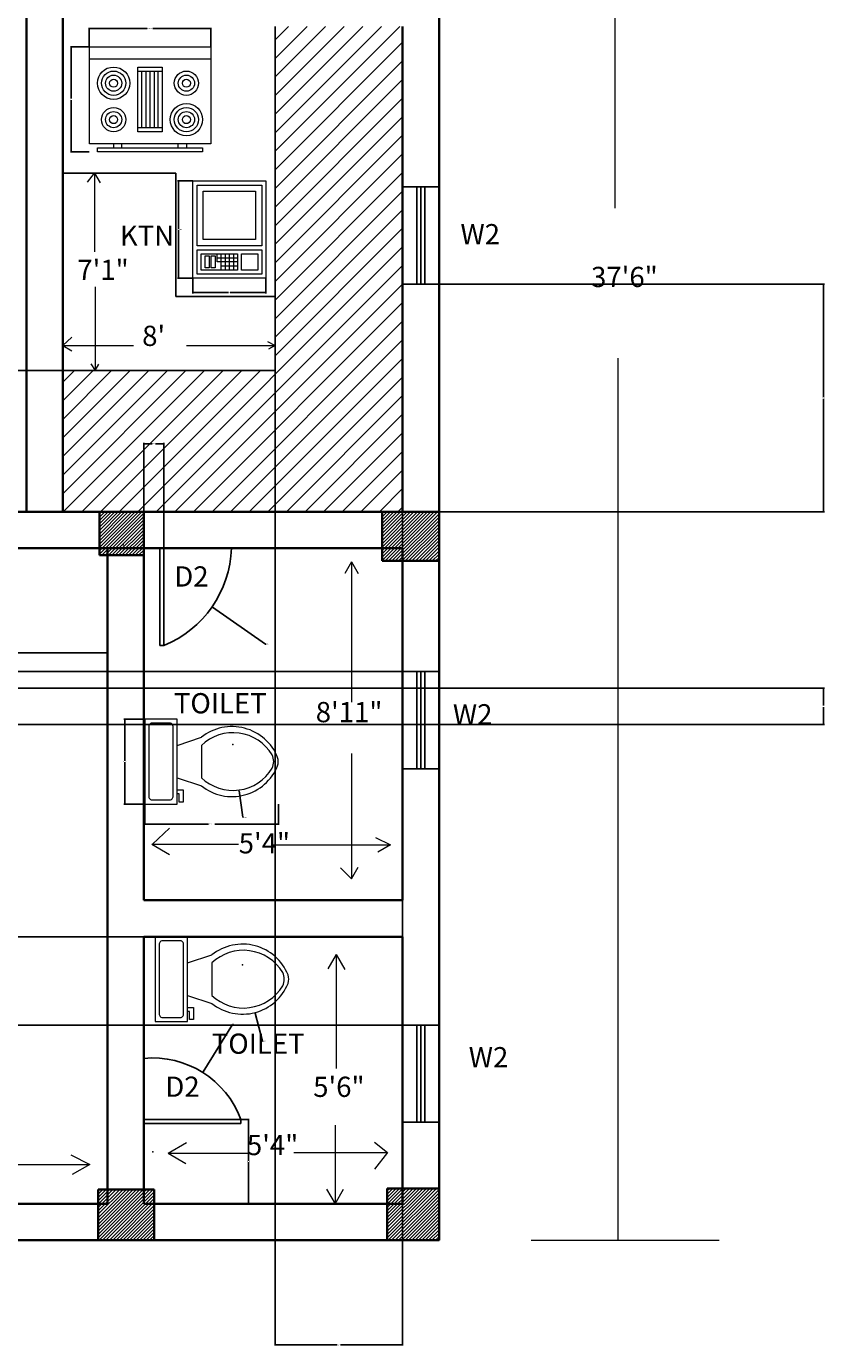
# Model space of a CAD drawing. Units: inches. Extents: x -4 to 429, y -457 to 84.
# Tile 3 of 4: x 232 to 429, y -457 to -131. Entities that reach past the tile are written whole.
import ezdxf

# ---------------------------------------------------------------- set-up
doc = ezdxf.new("R2010")
doc.units = ezdxf.units.IN
doc.header["$MEASUREMENT"] = 0
for name, color, linetype, lineweight in [('A-ANNO-DIMS', 2, 'Continuous', 18), ('A-ANNO-TEXT', 3, 'Continuous', 18), ('A-AREA-IDEN', 7, 'Continuous', 25), ('A-COLS', 7, 'Continuous', 35), ('A-COLS-PATT', 252, 'Continuous', 13), ('A-DOOR', 3, 'Continuous', 25), ('A-EQPM', 8, 'Continuous', 18), ('A-FLOR-CASE', 9, 'Continuous', 25), ('A-FLOR-CASE-PATT', 252, 'Continuous', 13), ('A-FLOR-FIXT', 9, 'Continuous', 18), ('A-GLAZ', 4, 'Continuous', 25), ('A-WALL', 7, 'Continuous', 35)]:
    doc.layers.add(name, color=color, linetype=linetype, lineweight=lineweight)
doc.styles.get("Standard").update_dxf_attribs({"font": 'arial.ttf'})
doc.dimstyles.get("Standard").update_dxf_attribs({"dimtxt": 0.18, "dimasz": 0.18, "dimexe": 0.18, "dimexo": 0.0625, "dimgap": 0.09, "dimtad": 0, "dimtih": 1, "dimtoh": 1, "dimdec": 4, "dimzin": 0, "dimdsep": 46, "dimtxsty": 'Standard', "dimcen": 0.09, "dimadec": 0, "dimazin": 0, "dimtfac": 1, "dimtdec": 4, "dimtofl": 0, "dimtmove": 0, "dimatfit": 3, "dimfxl": 1, "dimtolj": 1, "dimtzin": 0, "dimarcsym": 0})
pattern_1 = [(45, (-1330.13025, -719.5531), (-0.41542523, 0.41542523), [])]

# ---------------------------------------------------------------- blocks, each defined once
blk = doc.blocks.new('Microwave')
for p, q in [((18, 10), (22, 10)), ((19, 7), (19, 11)), ((20, 11), (20, 7)), ((21, 7), (21, 11)), ((22, 9), (18, 9)), ((18, 8), (22, 8)), ((22, 7), (18, 7)), ((19, 6), (19, 7)), ((20, 7), (20, 6)), ((20, 6), (18, 6))]:
    blk.add_line(p, q)
for points in [[(0, 0), (0, 18), (24, 18), (24, 0)], [(1, 1), (1, 17), (16, 17), (16, 1)], [(17, 1), (17, 17), (23, 17), (23, 1)], [(2.5, 2.5), (2.5, 15.5), (14.5, 15.5), (14.5, 2.5)], [(18, 12), (18, 16), (22, 16), (22, 12)], [(18, 2), (18, 11), (22, 11), (22, 2)], [(18.5, 4.5), (18.5, 5.5), (21.5, 5.5), (21.5, 4.5)], [(18.5, 3), (18.5, 4), (21.5, 4), (21.5, 3)]]:
    blk.add_lwpolyline(points, close=True)
blk = doc.blocks.new('Range-Oven - 30 in top')
for p, q in [((0, -3), (30, -3)), ((12, -6), (18, -6)), ((13, -20), (13, -6)), ((14, -6), (14, -20)), ((15, -20), (15, -6)), ((16, -6), (16, -20)), ((17, -20), (17, -6)), ((18, -20), (12, -20)), ((6, -24), (6, -25)), ((8, -25), (8, -24)), ((22, -25), (22, -24)), ((24, -24), (24, -25))]:
    blk.add_line(p, q)
for points in [[(0, -24), (0, 0), (30, 0), (30, -24)], [(12, -21), (12, -5), (18, -5), (18, -21)], [(2, -26), (2, -25), (28, -25), (28, -26)]]:
    blk.add_lwpolyline(points, close=True)
for centre, radius in [((6, -9), 4), ((6, -9), 3), ((24, -9), 3), ((6, -9), 2), ((6, -9), 1), ((24, -9), 2), ((24, -9), 1), ((6, -18), 3), ((6, -18), 2), ((24, -18), 4), ((24, -18), 3), ((24, -18), 2), ((6, -18), 1), ((24, -18), 1)]:
    blk.add_circle(centre, radius)
blk = doc.blocks.new('Toilet - top')
for p, q in [((9.5, -6), (9.5, -2)), ((-10, -8.5), (-8, -8.5)), ((-10, -9.5), (-10, -8.5)), ((-7, -9.5), (-10, -9.5)), ((-8, -8.5), (-8, -8)), ((-7, -8), (-7, -9.5)), ((-4, -8), (-6, -14)), ((4, -8), (6, -14)), ((4, -14), (-4, -14))]:
    blk.add_line(p, q)
blk.add_lwpolyline([(10.5, -8), (10.5, 0), (-10.5, 0), (-10.5, -8)], close=True)
for points in [[(-9.5, -2), (-9.5, -6)], [(8.5, -1), (-8.5, -1)], [(-8.5, -7), (8.5, -7)]]:
    blk.add_lwpolyline(points)
for centre, radius, start, end in [((-8.62, -1.88), 0.884, 81.8699, 188.1301), ((8.62, -1.88), 0.884, 351.8699, 98.1301), ((-8.62, -6.12), 0.884, 171.8699, 278.1301), ((8.62, -6.12), 0.884, 261.8699, 8.1301), ((3.52, -21.58), 12.17, 141.4691, 247.9714), ((4.2, -21.82), 11.33, 136.3677, 238.9468), ((-3.52, -21.58), 12.17, 292.0284, 38.5307), ((-4.2, -21.82), 11.33, 301.053, 43.6321), ((0, -27.88), 4, 245.7318, 294.2682), ((0, -29), 4, 254.8605, 285.1395)]:
    blk.add_arc(centre, radius, start, end)
blk = doc.blocks.new('WIN-24IN-9IN-WALL')
for p, q in [((0, 5.5), (24, 5.5)), ((0, 4.5), (24, 4.5)), ((0, 3.5), (24, 3.5))]:
    blk.add_line(p, q)
blk.add_lwpolyline([(0, 9), (24, 9), (24, 0), (0, 0)], close=True)
blk = doc.blocks.new('DOOR-LEAF-24IN')
for p, q in [((0, 0), (0, 24)), ((0, 24), (1, 24)), ((1, 24), (1, 0))]:
    blk.add_line(p, q)
blk = doc.blocks.new('*D20')
at = {"layer": 'A-ANNO-DIMS', "color": 0, "lineweight": -2, "transparency": 16777216}
for p, q in [((261.3, -323.62), (261.3, -328.69)), ((294.34, -323.62), (294.34, -328.69)), ((261.48, -328.51), (277.04, -328.51)), ((294.16, -328.51), (278.59, -328.51))]:
    blk.add_line(p, q, dxfattribs=at)
at = {"layer": 'A-ANNO-DIMS', "color": 0, "transparency": 16777216}
for points in [[(261.48, -328.48), (261.48, -328.54), (261.3, -328.51)], [(294.16, -328.48), (294.16, -328.54), (294.34, -328.51)]]:
    blk.add_solid(points, dxfattribs=at)
at = {"layer": 'Defpoints', "color": 0, "transparency": 16777216}
for p in [(261.3, -323.55), (294.34, -323.55), (261.3, -328.51)]:
    blk.add_point(p, dxfattribs=at)
at = {"layer": 'A-ANNO-DIMS', "color": 0, "transparency": 16777216, "insert": (277.82, -328.51), "char_height": 0.18, "attachment_point": 5}
blk.add_mtext('\\A1;WC 33 TYP.', dxfattribs=at)
blk = doc.blocks.new('*D21')
at = {"layer": 'A-ANNO-DIMS', "color": 0, "lineweight": -2, "transparency": 16777216}
for p, q in [((261.23, -302.55), (256.16, -302.55)), ((256.34, -302.73), (256.34, -312.87)), ((256.34, -323.37), (256.34, -313.24)), ((261.23, -323.55), (256.16, -323.55))]:
    blk.add_line(p, q, dxfattribs=at)
at = {"layer": 'A-ANNO-DIMS', "color": 0, "transparency": 16777216}
for points in [[(256.31, -302.73), (256.37, -302.73), (256.34, -302.55)], [(256.31, -323.37), (256.37, -323.37), (256.34, -323.55)]]:
    blk.add_solid(points, dxfattribs=at)
at = {"layer": 'Defpoints', "color": 0, "transparency": 16777216}
for p in [(256.34, -302.55), (261.3, -302.55), (261.3, -323.55)]:
    blk.add_point(p, dxfattribs=at)
at = {"layer": 'A-ANNO-DIMS', "color": 0, "transparency": 16777216, "insert": (256.34, -313.05), "char_height": 0.18, "attachment_point": 5}
blk.add_mtext('\\A1;21 TYP.', dxfattribs=at)
blk = doc.blocks.new('*D28')
at = {"layer": 'A-ANNO-DIMS', "color": 0, "lineweight": -2, "transparency": 16777216}
for p, q in [((273.16, -169.55), (269.44, -169.55)), ((269.62, -169.73), (269.62, -181.37)), ((269.62, -193.37), (269.62, -181.74)), ((273.16, -193.55), (269.44, -193.55))]:
    blk.add_line(p, q, dxfattribs=at)
at = {"layer": 'A-ANNO-DIMS', "color": 0, "transparency": 16777216}
for points in [[(269.59, -169.73), (269.65, -169.73), (269.62, -169.55)], [(269.59, -193.37), (269.65, -193.37), (269.62, -193.55)]]:
    blk.add_solid(points, dxfattribs=at)
at = {"layer": 'Defpoints', "color": 0, "transparency": 16777216}
for p in [(273.22, -169.55), (269.62, -193.55), (273.22, -193.55)]:
    blk.add_point(p, dxfattribs=at)
at = {"layer": 'A-ANNO-DIMS', "color": 0, "transparency": 16777216, "insert": (269.62, -181.55), "char_height": 0.18, "attachment_point": 5}
blk.add_mtext('\\A1;MICROWAVE 24', dxfattribs=at)
blk = doc.blocks.new('*D29')
at = {"layer": 'A-ANNO-DIMS', "color": 0, "lineweight": -2, "transparency": 16777216}
for p, q in [((273.22, -193.62), (273.22, -197.33)), ((291.22, -193.62), (291.22, -197.33)), ((273.4, -197.15), (282.01, -197.15)), ((291.04, -197.15), (282.43, -197.15))]:
    blk.add_line(p, q, dxfattribs=at)
at = {"layer": 'A-ANNO-DIMS', "color": 0, "transparency": 16777216}
for points in [[(273.4, -197.12), (273.4, -197.18), (273.22, -197.15)], [(291.04, -197.12), (291.04, -197.18), (291.22, -197.15)]]:
    blk.add_solid(points, dxfattribs=at)
at = {"layer": 'Defpoints', "color": 0, "transparency": 16777216}
for p in [(273.22, -193.55), (291.22, -193.55), (291.22, -197.15)]:
    blk.add_point(p, dxfattribs=at)
at = {"layer": 'A-ANNO-DIMS', "color": 0, "transparency": 16777216, "insert": (282.22, -197.15), "char_height": 0.18, "attachment_point": 5}
blk.add_mtext('\\A1;18', dxfattribs=at)
blk = doc.blocks.new('*D30')
at = {"layer": 'A-ANNO-DIMS', "color": 0, "lineweight": -2, "transparency": 16777216}
for p, q in [((247.6, -136.32), (247.6, -131.7)), ((247.78, -131.88), (261.91, -131.88)), ((277.42, -131.88), (263.3, -131.88)), ((277.6, -136.32), (277.6, -131.7))]:
    blk.add_line(p, q, dxfattribs=at)
at = {"layer": 'A-ANNO-DIMS', "color": 0, "transparency": 16777216}
for points in [[(247.78, -131.85), (247.78, -131.91), (247.6, -131.88)], [(277.42, -131.85), (277.42, -131.91), (277.6, -131.88)]]:
    blk.add_solid(points, dxfattribs=at)
at = {"layer": 'Defpoints', "color": 0, "transparency": 16777216}
for p in [(277.6, -131.88), (247.6, -136.38), (277.6, -136.38)]:
    blk.add_point(p, dxfattribs=at)
at = {"layer": 'A-ANNO-DIMS', "color": 0, "transparency": 16777216, "insert": (262.6, -131.88), "char_height": 0.18, "attachment_point": 5}
blk.add_mtext('\\A1;RANGE 30', dxfattribs=at)
blk = doc.blocks.new('*D31')
at = {"layer": 'A-ANNO-DIMS', "color": 0, "lineweight": -2, "transparency": 16777216}
for p, q in [((247.54, -136.38), (242.92, -136.38)), ((243.1, -136.56), (243.1, -149.2)), ((243.1, -162.2), (243.1, -149.57)), ((247.54, -162.38), (242.92, -162.38))]:
    blk.add_line(p, q, dxfattribs=at)
at = {"layer": 'A-ANNO-DIMS', "color": 0, "transparency": 16777216}
for points in [[(243.07, -136.56), (243.13, -136.56), (243.1, -136.38)], [(243.07, -162.2), (243.13, -162.2), (243.1, -162.38)]]:
    blk.add_solid(points, dxfattribs=at)
at = {"layer": 'Defpoints', "color": 0, "transparency": 16777216}
for p in [(243.1, -136.38), (247.6, -136.38), (247.6, -162.38)]:
    blk.add_point(p, dxfattribs=at)
at = {"layer": 'A-ANNO-DIMS', "color": 0, "transparency": 16777216, "insert": (243.1, -149.38), "char_height": 0.18, "attachment_point": 5}
blk.add_mtext('\\A1;26', dxfattribs=at)
blk = doc.blocks.new('*D33')
at = {"layer": 'A-ANNO-DIMS', "color": 0, "lineweight": -2, "transparency": 16777216}
for p, q in [((70.12, -294.9), (429.31, -294.9)), ((429.13, -295.08), (429.13, -299.22)), ((429.13, -303.72), (429.13, -299.59)), ((70.12, -303.9), (429.31, -303.9))]:
    blk.add_line(p, q, dxfattribs=at)
at = {"layer": 'A-ANNO-DIMS', "color": 0, "transparency": 16777216}
for points in [[(429.1, -295.08), (429.16, -295.08), (429.13, -294.9)], [(429.1, -303.72), (429.16, -303.72), (429.13, -303.9)]]:
    blk.add_solid(points, dxfattribs=at)
at = {"layer": 'Defpoints', "color": 0, "transparency": 16777216}
for p in [(70.06, -294.9), (70.06, -303.9), (429.13, -303.9)]:
    blk.add_point(p, dxfattribs=at)
at = {"layer": 'A-ANNO-DIMS', "color": 0, "transparency": 16777216, "insert": (429.13, -299.4), "char_height": 0.18, "attachment_point": 5}
blk.add_mtext('\\A1;9', dxfattribs=at)
blk = doc.blocks.new('*D36')
at = {"layer": 'A-ANNO-DIMS', "color": 0, "lineweight": -2, "transparency": 16777216}
for p, q in [((293.52, -131.4), (293.52, -457.42)), ((325.06, -131.4), (325.06, -457.42)), ((293.7, -457.24), (308.89, -457.24)), ((324.88, -457.24), (309.68, -457.24))]:
    blk.add_line(p, q, dxfattribs=at)
at = {"layer": 'A-ANNO-DIMS', "color": 0, "transparency": 16777216}
for points in [[(293.7, -457.21), (293.7, -457.27), (293.52, -457.24)], [(324.88, -457.21), (324.88, -457.27), (325.06, -457.24)]]:
    blk.add_solid(points, dxfattribs=at)
at = {"layer": 'Defpoints', "color": 0, "transparency": 16777216}
for p in [(293.52, -131.34), (325.06, -131.34), (325.06, -457.24)]:
    blk.add_point(p, dxfattribs=at)
at = {"layer": 'A-ANNO-DIMS', "color": 0, "transparency": 16777216, "insert": (309.29, -457.24), "char_height": 0.18, "attachment_point": 5}
blk.add_mtext('\\A1;31.54', dxfattribs=at)
blk = doc.blocks.new('*D37')
at = {"layer": 'A-ANNO-DIMS', "color": 0, "lineweight": -2, "transparency": 16777216}
for p, q in [((240.99, -216.42), (215.03, -216.42)), ((215.21, -216.6), (215.21, -233.7)), ((215.21, -251.16), (215.21, -234.06)), ((240.99, -251.34), (215.03, -251.34))]:
    blk.add_line(p, q, dxfattribs=at)
at = {"layer": 'A-ANNO-DIMS', "color": 0, "transparency": 16777216}
for points in [[(215.18, -216.6), (215.24, -216.6), (215.21, -216.42)], [(215.18, -251.16), (215.24, -251.16), (215.21, -251.34)]]:
    blk.add_solid(points, dxfattribs=at)
at = {"layer": 'Defpoints', "color": 0, "transparency": 16777216}
for p in [(215.21, -216.42), (241.06, -216.42), (241.06, -251.34)]:
    blk.add_point(p, dxfattribs=at)
at = {"layer": 'A-ANNO-DIMS', "color": 0, "transparency": 16777216, "insert": (215.21, -233.88), "char_height": 0.18, "attachment_point": 5}
blk.add_mtext('\\A1;34.92', dxfattribs=at)
blk = doc.blocks.new('*D40')
at = {"layer": 'A-ANNO-DIMS', "color": 0, "lineweight": -2, "transparency": 16777216}
for p, q in [((334.12, -195.04), (429.31, -195.04)), ((429.13, -195.22), (429.13, -223.01)), ((429.13, -251.16), (429.13, -223.37)), ((334.12, -251.34), (429.31, -251.34))]:
    blk.add_line(p, q, dxfattribs=at)
at = {"layer": 'A-ANNO-DIMS', "color": 0, "transparency": 16777216}
for points in [[(429.1, -195.22), (429.16, -195.22), (429.13, -195.04)], [(429.1, -251.16), (429.16, -251.16), (429.13, -251.34)]]:
    blk.add_solid(points, dxfattribs=at)
at = {"layer": 'Defpoints', "color": 0, "transparency": 16777216}
for p in [(334.06, -195.04), (334.06, -251.34), (429.13, -251.34)]:
    blk.add_point(p, dxfattribs=at)
at = {"layer": 'A-ANNO-DIMS', "color": 0, "transparency": 16777216, "insert": (429.13, -223.19), "char_height": 0.18, "attachment_point": 5}
blk.add_mtext('\\A1;56.3', dxfattribs=at)
blk = doc.blocks.new('*D41')
at = {"layer": 'A-ANNO-DIMS', "color": 0, "lineweight": -2, "transparency": 16777216}
for p, q in [((324.99, -260.34), (-3.97, -260.34)), ((-3.79, -260.52), (-3.79, -275.4)), ((-3.79, -290.65), (-3.79, -275.76)), ((324.99, -290.83), (-3.97, -290.83))]:
    blk.add_line(p, q, dxfattribs=at)
at = {"layer": 'A-ANNO-DIMS', "color": 0, "transparency": 16777216}
for points in [[(-3.82, -260.52), (-3.76, -260.52), (-3.79, -260.34)], [(-3.82, -290.65), (-3.76, -290.65), (-3.79, -290.83)]]:
    blk.add_solid(points, dxfattribs=at)
at = {"layer": 'Defpoints', "color": 0, "transparency": 16777216}
for p in [(325.06, -260.34), (-3.79, -290.83), (325.06, -290.83)]:
    blk.add_point(p, dxfattribs=at)
at = {"layer": 'A-ANNO-DIMS', "color": 0, "transparency": 16777216, "insert": (-3.79, -275.58), "char_height": 0.18, "attachment_point": 5}
blk.add_mtext('\\A1;30.486', dxfattribs=at)
blk = doc.blocks.new('*D42')
at = {"layer": 'A-ANNO-DIMS', "color": 0, "lineweight": -2, "transparency": 16777216}
for p, q in [((324.99, -356.34), (-3.97, -356.34)), ((-3.79, -356.52), (-3.79, -367.09)), ((-3.79, -378.03), (-3.79, -367.46)), ((324.99, -378.21), (-3.97, -378.21))]:
    blk.add_line(p, q, dxfattribs=at)
at = {"layer": 'A-ANNO-DIMS', "color": 0, "transparency": 16777216}
for points in [[(-3.82, -356.52), (-3.76, -356.52), (-3.79, -356.34)], [(-3.82, -378.03), (-3.76, -378.03), (-3.79, -378.21)]]:
    blk.add_solid(points, dxfattribs=at)
at = {"layer": 'Defpoints', "color": 0, "transparency": 16777216}
for p in [(325.06, -356.34), (-3.79, -378.21), (325.06, -378.21)]:
    blk.add_point(p, dxfattribs=at)
at = {"layer": 'A-ANNO-DIMS', "color": 0, "transparency": 16777216, "insert": (-3.79, -367.28), "char_height": 0.18, "attachment_point": 5}
blk.add_mtext('\\A1;21.87', dxfattribs=at)
blk = doc.blocks.new('*D48')
at = {"layer": 'A-ANNO-DIMS', "color": 0, "lineweight": -2, "transparency": 16777216}
for p, q in [((130.63, -260.4), (130.63, -286.37)), ((252.06, -260.4), (252.06, -286.37)), ((130.81, -286.19), (190.89, -286.19)), ((251.88, -286.19), (191.8, -286.19))]:
    blk.add_line(p, q, dxfattribs=at)
at = {"layer": 'A-ANNO-DIMS', "color": 0, "transparency": 16777216}
for points in [[(130.81, -286.16), (130.81, -286.22), (130.63, -286.19)], [(251.88, -286.16), (251.88, -286.22), (252.06, -286.19)]]:
    blk.add_solid(points, dxfattribs=at)
at = {"layer": 'Defpoints', "color": 0, "transparency": 16777216}
for p in [(130.63, -260.34), (252.06, -260.34), (130.63, -286.19)]:
    blk.add_point(p, dxfattribs=at)
at = {"layer": 'A-ANNO-DIMS', "color": 0, "transparency": 16777216, "insert": (191.35, -286.19), "char_height": 0.18, "attachment_point": 5}
blk.add_mtext('\\A1;121.42', dxfattribs=at)
blk = doc.blocks.new('*D49')
at = {"layer": 'A-ANNO-DIMS', "color": 0, "lineweight": -2, "transparency": 16777216}
for p, q in [((261.06, -260.28), (261.06, -234.31)), ((261.24, -234.49), (263.14, -234.49)), ((265.84, -234.49), (263.94, -234.49)), ((266.02, -260.28), (266.02, -234.31))]:
    blk.add_line(p, q, dxfattribs=at)
at = {"layer": 'A-ANNO-DIMS', "color": 0, "transparency": 16777216}
for points in [[(261.24, -234.46), (261.24, -234.52), (261.06, -234.49)], [(265.84, -234.46), (265.84, -234.52), (266.02, -234.49)]]:
    blk.add_solid(points, dxfattribs=at)
at = {"layer": 'Defpoints', "color": 0, "transparency": 16777216}
for p in [(266.02, -234.49), (261.06, -260.34), (266.02, -260.34)]:
    blk.add_point(p, dxfattribs=at)
at = {"layer": 'A-ANNO-DIMS', "color": 0, "transparency": 16777216, "insert": (263.54, -234.49), "char_height": 0.18, "attachment_point": 5}
blk.add_mtext('\\A1;4.964', dxfattribs=at)
blk = doc.blocks.new('*D50')
at = {"layer": 'A-ANNO-DIMS', "color": 0, "lineweight": -2, "transparency": 16777216}
for p, q in [((261.12, -401.49), (287.09, -401.49)), ((286.91, -401.67), (286.91, -411.73)), ((286.91, -422.16), (286.91, -412.1)), ((261.12, -422.34), (287.09, -422.34))]:
    blk.add_line(p, q, dxfattribs=at)
at = {"layer": 'A-ANNO-DIMS', "color": 0, "transparency": 16777216}
for points in [[(286.88, -401.67), (286.94, -401.67), (286.91, -401.49)], [(286.88, -422.16), (286.94, -422.16), (286.91, -422.34)]]:
    blk.add_solid(points, dxfattribs=at)
at = {"layer": 'Defpoints', "color": 0, "transparency": 16777216}
for p in [(261.06, -401.49), (261.06, -422.34), (286.91, -422.34)]:
    blk.add_point(p, dxfattribs=at)
at = {"layer": 'A-ANNO-DIMS', "color": 0, "transparency": 16777216, "insert": (286.91, -411.92), "char_height": 0.18, "attachment_point": 5}
blk.add_mtext('\\A1;20.848', dxfattribs=at)
blk = doc.blocks.new('*D57')
at = {"layer": 'A-ANNO-DIMS', "color": 0, "lineweight": -2, "transparency": 16777216}
for p, q in [((255.86, -259.49), (256.04, -259.49)), ((255.95, -259.58), (255.95, -259.4)), ((291.14, -284.02), (278.09, -274.92)), ((291.32, -284.02), (291.14, -284.02))]:
    blk.add_line(p, q, dxfattribs=at)
at = {"layer": 'A-ANNO-DIMS', "color": 0, "transparency": 16777216}
blk.add_solid([(278.11, -274.9), (278.07, -274.95), (277.94, -274.82)], dxfattribs=at)
at = {"layer": 'Defpoints', "color": 0, "transparency": 16777216}
for p in [(255.95, -259.49), (277.94, -274.82)]:
    blk.add_point(p, dxfattribs=at)
at = {"layer": 'A-ANNO-DIMS', "color": 0, "transparency": 16777216, "insert": (291.79, -284.02), "char_height": 0.18, "attachment_point": 5}
blk.add_mtext('\\A1;R26.81', dxfattribs=at)
blk = doc.blocks.new('*D58')
at = {"layer": 'A-ANNO-DIMS', "color": 0, "lineweight": -2, "transparency": 16777216}
for p, q in [((283.03, -378.07), (275.72, -389.72)), ((283.21, -378.07), (283.03, -378.07)), ((263.18, -409.54), (263.36, -409.54)), ((263.27, -409.63), (263.27, -409.45))]:
    blk.add_line(p, q, dxfattribs=at)
at = {"layer": 'A-ANNO-DIMS', "color": 0, "transparency": 16777216}
blk.add_solid([(275.69, -389.7), (275.74, -389.74), (275.62, -389.87)], dxfattribs=at)
at = {"layer": 'Defpoints', "color": 0, "transparency": 16777216}
for p in [(275.62, -389.87), (263.27, -409.54)]:
    blk.add_point(p, dxfattribs=at)
at = {"layer": 'A-ANNO-DIMS', "color": 0, "transparency": 16777216, "insert": (283.69, -378.07), "char_height": 0.18, "attachment_point": 5}
blk.add_mtext('\\A1;R23.23', dxfattribs=at)
blk = doc.blocks.new('*D62')
at = {"layer": 'A-ANNO-DIMS', "color": 0, "lineweight": -2, "transparency": 16777216}
for p, q in [((285.38, -363.32), (285.56, -363.32)), ((285.47, -363.41), (285.47, -363.23)), ((290.41, -382.15), (288.6, -375.26)), ((290.59, -382.15), (290.41, -382.15))]:
    blk.add_line(p, q, dxfattribs=at)
at = {"layer": 'A-ANNO-DIMS', "color": 0, "transparency": 16777216}
blk.add_solid([(288.63, -375.26), (288.58, -375.27), (288.56, -375.09)], dxfattribs=at)
at = {"layer": 'Defpoints', "color": 0, "transparency": 16777216}
for p in [(285.47, -363.32), (288.56, -375.09)]:
    blk.add_point(p, dxfattribs=at)
at = {"layer": 'A-ANNO-DIMS', "color": 0, "transparency": 16777216, "insert": (291.27, -382.15), "char_height": 0.18, "attachment_point": 5}
blk.add_mtext('\\A1;4X R12.17', dxfattribs=at)
blk = doc.blocks.new('*D63')
at = {"layer": 'A-ANNO-DIMS', "color": 0, "lineweight": -2, "transparency": 16777216}
for p, q in [((283.02, -308.85), (283.2, -308.85)), ((283.11, -308.94), (283.11, -308.76)), ((285.53, -326.82), (284.65, -320.26)), ((285.71, -326.82), (285.53, -326.82))]:
    blk.add_line(p, q, dxfattribs=at)
at = {"layer": 'A-ANNO-DIMS', "color": 0, "transparency": 16777216}
blk.add_solid([(284.68, -320.26), (284.62, -320.27), (284.62, -320.08)], dxfattribs=at)
at = {"layer": 'Defpoints', "color": 0, "transparency": 16777216}
for p in [(283.11, -308.85), (284.62, -320.08)]:
    blk.add_point(p, dxfattribs=at)
at = {"layer": 'A-ANNO-DIMS', "color": 0, "transparency": 16777216, "insert": (286.39, -326.82), "char_height": 0.18, "attachment_point": 5}
blk.add_mtext('\\A1;4X R11.33', dxfattribs=at)

msp = doc.modelspace()

# ---------------------------------------------------------------- hatches: boundary and pattern name
at = {"layer": 'A-COLS-PATT'}
h = msp.add_hatch(dxfattribs=at)
h.set_pattern_fill('ANSI31', color=256, scale=4.7)
h.set_pattern_definition(pattern_1)
h.paths.add_polyline_path([(334.0572, -251.3399), (325.0572, -251.3399), (319.9964, -251.3399), (319.9964, -260.3399), (325.0572, -260.3399), (325.0572, -263.4636), (334.0572, -263.4636)])
h.paths.add_polyline_path([(325.0572, -260.3399), (319.9964, -260.3399), (319.9964, -263.4636), (325.0572, -263.4636)], flags=17)
h.paths.add_polyline_path([(34.0899, -251.3399), (31.0572, -251.3399), (22.0572, -251.3399), (22.0572, -263.5568), (31.0572, -263.5568), (31.0572, -260.3399), (34.0899, -260.3399)])
h.paths.add_polyline_path([(34.0899, -260.3399), (31.0572, -260.3399), (31.0572, -263.5568), (34.0899, -263.5568)], flags=17)
h = msp.add_hatch(dxfattribs=at)
h.set_pattern_fill('ANSI31', color=256, scale=4.7)
h.set_pattern_definition(pattern_1)
h.paths.add_polyline_path([(261.0572, -251.3399), (250.1046, -251.3399), (250.1046, -260.3399), (261.0572, -260.3399)])
h.paths.add_polyline_path([(252.0572, -260.3399), (250.1046, -260.3399), (250.1046, -262.0762), (252.0572, -262.0762)])
h.paths.add_polyline_path([(261.0572, -260.3399), (252.0572, -260.3399), (252.0572, -262.0762), (261.0572, -262.0762)])
h = msp.add_hatch(dxfattribs=at)
h.set_pattern_fill('ANSI31', color=256, scale=4.7)
h.set_pattern_definition(pattern_1)
h.paths.add_polyline_path([(263.6379, -422.3399), (261.0572, -422.3399), (261.0572, -418.8132), (252.0572, -418.8132), (252.0572, -422.3399), (249.7857, -422.3399), (249.7857, -431.3399), (263.6379, -431.3399)])
h.paths.add_polyline_path([(252.0572, -418.8132), (249.7857, -418.8132), (249.7857, -422.3399), (252.0572, -422.3399)], flags=17)
h.paths.add_polyline_path([(263.6379, -418.8132), (261.0572, -418.8132), (261.0572, -422.3399), (263.6379, -422.3399)], flags=17)
h = msp.add_hatch(dxfattribs=at)
h.set_pattern_fill('ANSI31', color=256, scale=4.7)
h.set_pattern_definition(pattern_1)
h.paths.add_polyline_path([(325.0572, -418.5798), (321.2689, -418.5798), (321.2689, -422.3399), (325.0572, -422.3399)], flags=17)
h.paths.add_polyline_path([(334.0572, -418.5798), (325.0572, -418.5798), (325.0572, -422.3399), (321.2689, -422.3399), (321.2689, -431.3399), (334.0572, -431.3399)])
at = {"layer": 'A-FLOR-CASE-PATT'}
h = msp.add_hatch(dxfattribs=at)
h.set_pattern_fill('ANSI31', color=256, scale=26)
h.set_pattern_definition([(45, (-1330.1303, -719.553), (-2.298097, 2.298097), [])])
h.paths.add_polyline_path([(325.0572, -131.3399), (293.5167, -131.3399), (293.5167, -216.4188), (241.0572, -216.4188), (241.0572, -251.3399), (325.0572, -251.3399)])

# ---------------------------------------------------------------- linework, layer by layer
at = {"layer": 'A-ANNO-DIMS'}
for p, q in [((377.4887, 18.6601), (377.4887, -176.2694)), ((247.1193, -169.8571), (248.9197, -167.5973)), ((248.9197, -167.5973), (248.9197, -187.0745)), ((248.9197, -167.5973), (250.3069, -169.9999)), ((249.0695, -195.7353), (249.0695, -216.4188)), ((243.2479, -208.1928), (241.0572, -210.2098)), ((241.0572, -210.2098), (258.5297, -210.2098)), ((241.0572, -210.2098), (243.3025, -211.5061)), ((271.5893, -210.2098), (293.5167, -210.2098)), ((291.6293, -209.2601), (293.5167, -210.2098)), ((293.5167, -210.2098), (291.88, -211.1548)), ((247.9929, -214.7252), (249.0695, -216.4188)), ((249.0695, -216.4188), (249.9759, -214.8489)), ((378.2756, -213.3463), (378.2756, -431.3399)), ((312.4369, -263.6991), (310.7836, -266.5628)), ((312.4369, -263.6991), (312.4369, -298.3746)), ((312.4369, -263.6991), (314.0927, -266.567)), ((312.4369, -311.0802), (312.4369, -342.0499)), ((263.1937, -333.4878), (267.3935, -329.4934)), ((318.3203, -331.8236), (322.0243, -333.6537)), ((263.0687, -333.4878), (284.492, -333.4878)), ((263.0687, -333.4878), (267.4223, -336.0013)), ((292.6296, -333.6537), (322.0243, -333.6537)), ((322.0243, -333.6537), (318.9595, -335.4231)), ((309.701, -339.3156), (312.4369, -342.0499)), ((312.4369, -342.0499), (314.0884, -339.1895)), ((308.6569, -360.748), (306.6025, -364.3063)), ((308.6569, -360.748), (308.6569, -388.8905)), ((308.6569, -360.748), (310.7932, -364.4481)), ((308.386, -402.9617), (308.386, -422.3399)), ((267.062, -409.8655), (271.6342, -407.2257)), ((318.1218, -407.1378), (321.3323, -409.6606)), ((243.0363, -410.2286), (247.6925, -412.6439)), ((267.062, -409.8655), (286.861, -409.8655)), ((267.062, -409.8655), (271.4469, -412.3971)), ((298.1349, -409.6606), (321.3323, -409.6606)), ((321.3323, -409.6606), (318.1018, -413.7716)), ((198.9877, -412.6439), (247.6925, -412.6439)), ((247.6925, -412.6439), (243.3818, -415.1326)), ((306.2357, -418.7619), (308.386, -422.3399)), ((308.386, -422.3399), (310.4388, -418.7843)), ((356.7945, -431.3861), (403.2831, -431.3861))]:
    msp.add_line(p, q, dxfattribs=at)
at = {"layer": 'A-COLS'}
for p, q in [((261.0572, -251.3399), (250.1046, -251.3399)), ((250.1046, -251.3399), (250.1046, -262.0762)), ((261.0572, -260.3399), (261.0572, -251.3399)), ((319.9964, -263.4636), (319.9964, -251.3399)), ((325.0572, -251.3399), (334.0572, -251.3399)), ((250.1046, -262.0762), (261.0572, -262.0762)), ((319.9964, -263.4636), (334.0572, -263.4636)), ((249.7857, -431.3399), (249.7857, -418.8132)), ((249.7857, -418.8132), (263.6379, -418.8132)), ((263.6379, -418.8132), (263.6379, -431.3399)), ((334.0572, -418.5798), (321.2689, -418.5798)), ((321.2689, -418.5798), (321.2689, -431.3399))]:
    msp.add_line(p, q, dxfattribs=at)
at = {"layer": 'A-DOOR'}
for centre, radius, start, end in [((255.9463, -259.4939), 26.8112, 292.073261, 358.191774), ((263.2693, -409.5429), 23.2277, 20.279231, 95.464723)]:
    msp.add_arc(centre, radius, start, end, dxfattribs=at)
at = {"layer": 'A-FLOR-CASE'}
for p, q in [((293.5167, -131.3399), (293.5167, -216.4188)), ((241.0572, -167.5973), (268.9792, -167.5973)), ((268.9792, -167.5973), (268.9792, -198.1317)), ((268.9792, -198.1317), (293.5167, -198.1317)), ((293.5167, -216.4188), (241.0572, -216.4188))]:
    msp.add_line(p, q, dxfattribs=at)
at = {"layer": 'A-WALL'}
for p, q in [((232.0572, -251.3399), (232.0572, -122.3399)), ((241.0572, -251.3399), (241.0572, -122.3399)), ((325.0572, -131.3399), (325.0572, -251.3399)), ((31.0572, -251.3399), (325.0572, -251.3399)), ((31.0572, -260.3399), (325.0572, -260.3399)), ((252.0572, -260.3399), (252.0572, -422.3399)), ((261.0572, -260.3399), (261.0572, -347.3399)), ((325.0572, -260.3399), (325.0572, -347.3399)), ((325.0572, -347.3399), (261.0572, -347.3399)), ((325.0572, -356.3399), (261.0572, -356.3399)), ((261.0572, -356.3399), (261.0572, -422.3399)), ((325.0572, -356.3399), (325.0572, -422.3399)), ((252.0572, -422.3399), (118.0572, -422.3399)), ((325.0572, -422.3399), (261.0572, -422.3399))]:
    msp.add_line(p, q, dxfattribs=at)
msp.add_lwpolyline([(22.0572, 18.6601), (334.0572, 18.6601), (334.0572, -431.3399), (22.0572, -431.3399)], close=True, dxfattribs=at)

# ---------------------------------------------------------------- block references
at = {"layer": 'A-DOOR'}
for p, rotation in [((266.0219, -260.3398), 180), ((261.0571, -401.492), 270)]:
    msp.add_blockref('DOOR-LEAF-24IN', p, dxfattribs=dict(at, rotation=rotation))
at = {"layer": 'A-EQPM'}
msp.add_blockref('Range-Oven - 30 in top', (247.6038, -136.3834), dxfattribs=at)
at = {"layer": 'A-EQPM', "rotation": 270}
msp.add_blockref('Microwave', (273.2213, -169.5549), dxfattribs=at)
at = {"layer": 'A-FLOR-FIXT', "rotation": 90}
for p in [(261.2956, -313.0548), (263.8863, -366.8399)]:
    msp.add_blockref('Toilet - top', p, dxfattribs=at)
at = {"layer": 'A-GLAZ', "extrusion": (0, 0, -1), "zscale": -1, "rotation": 269.9999999999999}
for p in [(-334.0573, -171.0372), (-334.0573, -290.8262), (-334.0573, -378.2116)]:
    msp.add_blockref('WIN-24IN-9IN-WALL', p, dxfattribs=at)

# ---------------------------------------------------------------- texts
at = {"layer": 'A-ANNO-DIMS', "char_height": 5, "attachment_point": 1}
for s, width, insert in [('7\'1"', 10.199223, (244.6362, -189.005)), ('37\'6"', 41.64508, (371.6297, -190.7711)), ("8'", 8.637028, (260.6635, -205.3302)), ('8\'11"', 24.986994, (303.5702, -298.3262)), ('5\'4"', 21.398917, (284.5226, -330.755)), ('5\'6"', 9.063832, (302.9437, -390.9482)), ('5\'4"', 7.901802, (286.559, -405.3405))]:
    msp.add_mtext_dynamic_manual_height_columns(s, width=width, gutter_width=25, heights=[0], dxfattribs=dict(at, insert=insert))
at = {"layer": 'A-ANNO-TEXT', "char_height": 5, "attachment_point": 1}
for s, width, insert in [('W2', 35.907088, (339.3492, -180.2029)), ('D2', 7.372865, (268.6029, -264.8038)), ('W2', 9.913025, (337.4774, -298.8735)), ('W2', 22.674394, (341.3957, -383.6316)), ('D2', 6.583052, (266.3915, -390.9186))]:
    msp.add_mtext_dynamic_manual_height_columns(s, width=width, gutter_width=25, heights=[0], dxfattribs=dict(at, insert=insert))
at = {"layer": 'A-AREA-IDEN', "char_height": 5, "attachment_point": 1}
for s, width, insert in [('KTN', 7.218497, (255.1568, -180.5565)), ('TOILET', 35.485263, (268.4995, -296.1384)), ('TOILET', 20.609834, (277.863, -380.2864))]:
    msp.add_mtext_dynamic_manual_height_columns(s, width=width, gutter_width=25, heights=[0], dxfattribs=dict(at, insert=insert))

# ---------------------------------------------------------------- dimensions: what is measured, and where the dimension line sits
at = {"layer": 'A-ANNO-DIMS'}
dim = msp.add_linear_dim(base=(277.6038, -131.8834), p1=(247.6038, -136.3834), p2=(277.6038, -136.3834), text='RANGE <>', dimstyle='Standard', override={"dimdec": 0, "dimlfac": 1, "dimrnd": 0, "dimzin": 0, "dimdsep": 46, "dimlunit": 2}, dxfattribs=at)
dim.commit()
dim.dimension.update_dxf_attribs({"geometry": '*D30', "text_midpoint": (262.6038, -131.8834)})
for base, p1, p2, override, picture, middle in [((325.0572, -457.2361), (293.5167, -131.3399), (325.0572, -131.3399), {"dimdec": 2, "dimlfac": 1, "dimrnd": 0, "dimzin": 0, "dimdsep": 46, "dimlunit": 2}, '*D36', (309.287, -457.2361)), ((291.2213, -197.1549), (273.2213, -193.5549), (291.2213, -193.5549), {"dimdec": 0, "dimlfac": 1, "dimrnd": 0, "dimzin": 0, "dimdsep": 46, "dimlunit": 2}, '*D29', (282.2213, -197.1549))]:
    dim = msp.add_linear_dim(base=base, p1=p1, p2=p2, dimstyle='Standard', override=override, dxfattribs=at)
    dim.commit()
    dim.dimension.update_dxf_attribs({"geometry": picture, "text_midpoint": middle})
for base, p1, p2, angle, override, picture, middle in [((243.1038, -136.3834), (247.6038, -162.3834), (247.6038, -136.3834), 90, {"dimdec": 0, "dimlfac": 1, "dimrnd": 0, "dimzin": 0, "dimdsep": 46, "dimlunit": 2}, '*D31', (243.1038, -149.3834)), ((429.1331, -251.3399), (334.0572, -195.037), (334.0572, -251.3399), 90, {"dimdec": 1, "dimlfac": 1, "dimrnd": 0, "dimzin": 0, "dimdsep": 46, "dimlunit": 2}, '*D40', (429.1331, -223.1885)), ((215.2072, -216.4188), (241.0572, -251.3399), (241.0572, -216.4188), 90, {"dimdec": 2, "dimlfac": 1, "dimrnd": 0, "dimzin": 0, "dimdsep": 46, "dimlunit": 2}, '*D37', (215.2072, -233.8794)), ((266.02169, -234.4899), (261.05724, -260.3399), (266.02169, -260.3399), 0, {"dimdec": 3, "dimlfac": 1, "dimrnd": 0, "dimzin": 0, "dimdsep": 46, "dimlunit": 2}, '*D49', (263.53946, -234.4899)), ((-3.7928, -290.8261), (325.0572, -260.3399), (325.0572, -290.8261), 90, {"dimdec": 3, "dimlfac": 1, "dimrnd": 0, "dimzin": 0, "dimdsep": 46, "dimlunit": 2}, '*D41', (-3.7928, -275.583)), ((130.6339, -286.1899), (252.0572, -260.3399), (130.6339, -260.3399), 180, {"dimdec": 2, "dimlfac": 1, "dimrnd": 0, "dimzin": 0, "dimdsep": 46, "dimlunit": 2}, '*D48', (191.3455, -286.1899)), ((429.1331, -303.9035), (70.0572, -294.9035), (70.0572, -303.9035), 90, {"dimdec": 0, "dimlfac": 1, "dimrnd": 0, "dimzin": 0, "dimdsep": 46, "dimlunit": 2}, '*D33', (429.1331, -299.4035)), ((-3.7928, -378.2115), (325.0572, -356.3399), (325.0572, -378.2115), 90, {"dimdec": 2, "dimlfac": 1, "dimrnd": 0, "dimzin": 0, "dimdsep": 46, "dimlunit": 2}, '*D42', (-3.7928, -367.2757)), ((286.9072, -422.3399), (261.0572, -401.4922), (261.0572, -422.3399), 270, {"dimdec": 3, "dimlfac": 1, "dimrnd": 0, "dimzin": 0, "dimdsep": 46, "dimlunit": 2}, '*D50', (286.9072, -411.9161))]:
    dim = msp.add_linear_dim(base=base, p1=p1, p2=p2, angle=angle, dimstyle='Standard', override=override, dxfattribs=at)
    dim.commit()
    dim.dimension.update_dxf_attribs({"geometry": picture, "text_midpoint": middle})
for base, p1, p2, angle, text, picture, middle in [((269.6213, -193.5549), (273.2213, -169.5549), (273.2213, -193.5549), 270, 'MICROWAVE <>', '*D28', (269.6213, -181.5549)), ((256.3386, -302.5548), (261.2956, -323.5548), (261.2956, -302.5548), 90, '<> TYP.', '*D21', (256.3386, -313.0548)), ((261.2956, -328.5118), (294.3418, -323.5548), (261.2956, -323.5548), 180, 'WC <> TYP.', '*D20', (277.8187, -328.5118))]:
    dim = msp.add_linear_dim(base=base, p1=p1, p2=p2, angle=angle, text=text, dimstyle='Standard', override={"dimdec": 0, "dimlfac": 1, "dimrnd": 0, "dimzin": 0, "dimdsep": 46, "dimlunit": 2}, dxfattribs=at)
    dim.commit()
    dim.dimension.update_dxf_attribs({"geometry": picture, "text_midpoint": middle})
for center, mpoint, picture, middle in [((255.9463, -259.4939), (277.9443, -274.8212), '*D57', (291.7855, -284.0176)), ((263.2693, -409.5429), (275.622, -389.8721), '*D58', (283.6934, -378.0696))]:
    dim = msp.add_radius_dim(center=center, mpoint=mpoint, dimstyle='Standard', override={"dimdec": 2, "dimlfac": 1, "dimrnd": 0, "dimzin": 0, "dimdsep": 46, "dimlunit": 2}, dxfattribs=at)
    dim.commit()
    dim.dimension.update_dxf_attribs({"geometry": picture, "text_midpoint": middle, "dimtype": 164})
for center, mpoint, picture, middle in [((283.113, -308.8549), (284.623, -320.083), '*D63', (286.3859, -326.8198)), ((285.4668, -363.3203), (288.559, -375.0899), '*D62', (291.2711, -382.1517))]:
    dim = msp.add_radius_dim(center=center, mpoint=mpoint, text='4X <>', dimstyle='Standard', override={"dimdec": 2, "dimlfac": 1, "dimrnd": 0, "dimzin": 0, "dimdsep": 46, "dimlunit": 2}, dxfattribs=at)
    dim.commit()
    dim.dimension.update_dxf_attribs({"geometry": picture, "text_midpoint": middle, "dimtype": 164})

doc.saveas('drawing.dxf')
